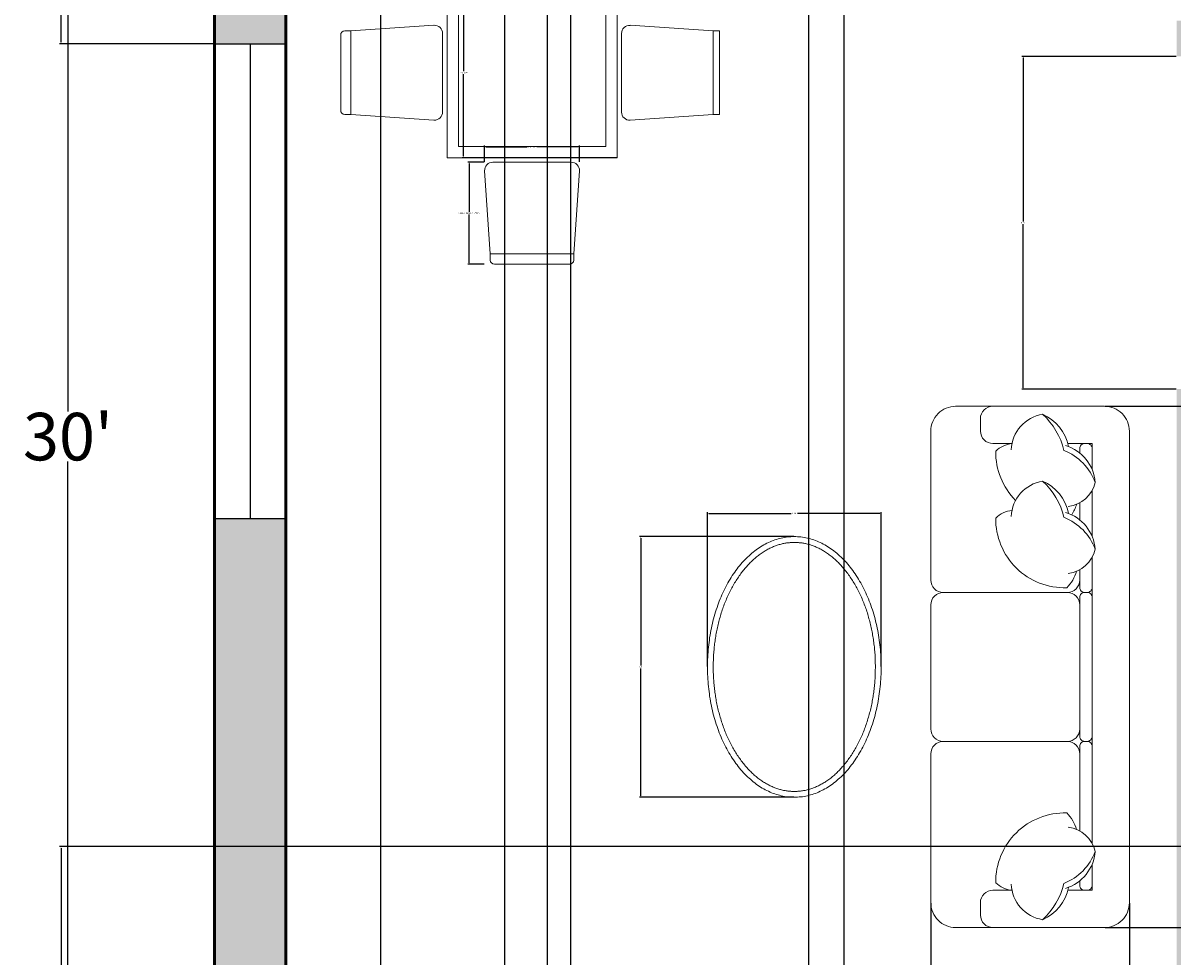
# Model space of a CAD drawing. Units: inches. Extents: x -2 to 282, y -370 to 35.
# Tile 2 of 5: x -2 to 143, y -237 to -119. Entities that reach past the tile are written whole.
import ezdxf

# ---------------------------------------------------------------- set-up
doc = ezdxf.new("R2010")
doc.units = ezdxf.units.IN
doc.header["$MEASUREMENT"] = 0
for name, color, linetype, lineweight in [('A-ANNO-DIMS', 2, 'Continuous', 18), ('A-FURN', 8, 'Continuous', 18), ('A-GLAZ', 4, 'Continuous', 25), ('A-WALL', 7, 'Continuous', 50), ('A-WALL-PATT', 252, 'Continuous', 13)]:
    doc.layers.add(name, color=color, linetype=linetype, lineweight=lineweight)
doc.styles.get("Standard").update_dxf_attribs({"font": 'arial.ttf'})
doc.dimstyles.get("Standard").update_dxf_attribs({"dimtxt": 0.18, "dimasz": 0.18, "dimexe": 0.18, "dimexo": 0.0625, "dimgap": 0.09, "dimtad": 0, "dimtih": 1, "dimtoh": 1, "dimdec": 0, "dimzin": 0, "dimdsep": 46, "dimlunit": 3, "dimtxsty": 'Standard', "dimcen": 0.09, "dimadec": 0, "dimazin": 0, "dimtfac": 1, "dimtdec": 0, "dimtofl": 0, "dimtmove": 0, "dimatfit": 3, "dimfxl": 1, "dimtolj": 1, "dimtzin": 0, "dimarcsym": 0})

# ---------------------------------------------------------------- blocks, each defined once
blk = doc.blocks.new('*D2')
at = {"layer": 'A-ANNO-DIMS', "color": 0, "lineweight": -2, "transparency": 16777216}
for p, q in [((22.35, 9.19), (3.74, 9.19)), ((3.92, 9.01), (3.92, -167.65)), ((3.92, -350.63), (3.92, -173.97)), ((22.35, -350.81), (3.74, -350.81))]:
    blk.add_line(p, q, dxfattribs=at)
at = {"layer": 'A-ANNO-DIMS', "color": 0, "transparency": 16777216}
for points in [[(3.89, 9.01), (3.95, 9.01), (3.92, 9.19)], [(3.89, -350.63), (3.95, -350.63), (3.92, -350.81)]]:
    blk.add_solid(points, dxfattribs=at)
at = {"layer": 'Defpoints', "color": 0, "transparency": 16777216}
for p in [(3.92, 9.19), (22.41, 9.19), (22.41, -350.81)]:
    blk.add_point(p, dxfattribs=at)
at = {"layer": 'A-ANNO-DIMS', "color": 0, "transparency": 16777216, "insert": (3.92, -170.81), "char_height": 6, "attachment_point": 5}
blk.add_mtext("\\A1;30'", dxfattribs=at)
blk = doc.blocks.new('WINDOW-60IN')
for p, q in [((0, 0), (0, 60)), ((0, 60), (9, 60)), ((4.5, 60), (4.5, 0)), ((9, 60), (9, 0)), ((9, 0), (0, 0))]:
    blk.add_line(p, q)
blk = doc.blocks.new('DINING-CHAIR')
for p, q in [((0.71, 12.36), (0.71, 11.58)), ((10.75, 12.87), (1.23, 12.87)), ((11.26, 11.58), (11.26, 12.36)), ((0, 1.09), (0.71, 11.58)), ((11.26, 11.58), (0.71, 11.58)), ((11.26, 11.58), (11.98, 1.09)), ((1.03, 0), (10.95, 0))]:
    blk.add_line(p, q)
for centre, radius, start, end in [((1.23, 12.36), 0.515, 90, 180), ((10.75, 12.36), 0.515, 0, 90), ((1.03, 1.03), 1.03, 176.8779, 270), ((10.95, 1.03), 1.03, 270, 3.1221)]:
    blk.add_arc(centre, radius, start, end)
blk = doc.blocks.new('*D15')
at = {"layer": 'A-ANNO-DIMS', "color": 0, "lineweight": -2, "transparency": 16777216}
for p, q in [((56.46, -136.16), (54.41, -136.16)), ((54.59, -136.34), (54.59, -142.42)), ((54.59, -148.86), (54.59, -142.78)), ((56.46, -149.04), (54.41, -149.04))]:
    blk.add_line(p, q, dxfattribs=at)
at = {"layer": 'A-ANNO-DIMS', "color": 0, "transparency": 16777216}
for points in [[(54.56, -136.34), (54.62, -136.34), (54.59, -136.16)], [(54.56, -148.86), (54.62, -148.86), (54.59, -149.04)]]:
    blk.add_solid(points, dxfattribs=at)
at = {"layer": 'Defpoints', "color": 0, "transparency": 16777216}
for p in [(56.52, -136.16), (54.59, -149.04), (56.52, -149.04)]:
    blk.add_point(p, dxfattribs=at)
at = {"layer": 'A-ANNO-DIMS', "color": 0, "transparency": 16777216, "insert": (54.59, -142.6), "char_height": 0.18, "attachment_point": 5}
blk.add_mtext('\\A1;DINING CHAIR 1\'-1" TYP.', dxfattribs=at)
blk = doc.blocks.new('*D16')
at = {"layer": 'A-ANNO-DIMS', "color": 0, "lineweight": -2, "transparency": 16777216}
for p, q in [((56.52, -136.1), (56.52, -134.05)), ((56.7, -134.23), (61.9, -134.23)), ((68.35, -134.23), (63.16, -134.23)), ((68.53, -136.1), (68.53, -134.05))]:
    blk.add_line(p, q, dxfattribs=at)
at = {"layer": 'A-ANNO-DIMS', "color": 0, "transparency": 16777216}
for points in [[(56.7, -134.2), (56.7, -134.26), (56.52, -134.23)], [(68.35, -134.2), (68.35, -134.26), (68.53, -134.23)]]:
    blk.add_solid(points, dxfattribs=at)
at = {"layer": 'Defpoints', "color": 0, "transparency": 16777216}
for p in [(56.52, -134.23), (56.52, -136.16), (68.53, -136.16)]:
    blk.add_point(p, dxfattribs=at)
at = {"layer": 'A-ANNO-DIMS', "color": 0, "transparency": 16777216, "insert": (62.53, -134.23), "char_height": 0.18, "attachment_point": 5}
blk.add_mtext('\\A1;1\'-0" TYP.', dxfattribs=at)
blk = doc.blocks.new('*D30')
at = {"layer": 'A-ANNO-DIMS', "color": 0, "lineweight": -2, "transparency": 16777216}
for p, q in [((22.35, -71.81), (2.86, -71.81)), ((3.04, -71.99), (3.04, -96.32)), ((3.04, -121.02), (3.04, -96.69)), ((22.35, -121.2), (2.86, -121.2))]:
    blk.add_line(p, q, dxfattribs=at)
at = {"layer": 'A-ANNO-DIMS', "color": 0, "transparency": 16777216}
for points in [[(3.01, -71.99), (3.07, -71.99), (3.04, -71.81)], [(3.01, -121.02), (3.07, -121.02), (3.04, -121.2)]]:
    blk.add_solid(points, dxfattribs=at)
at = {"layer": 'Defpoints', "color": 0, "transparency": 16777216}
for p in [(22.41, -71.81), (3.04, -121.2), (22.41, -121.2)]:
    blk.add_point(p, dxfattribs=at)
at = {"layer": 'A-ANNO-DIMS', "color": 0, "transparency": 16777216, "insert": (3.04, -96.51), "char_height": 0.18, "attachment_point": 5}
blk.add_mtext('\\A1;4\'-1 1/2"', dxfattribs=at)
blk = doc.blocks.new('*D37')
at = {"layer": 'A-ANNO-DIMS', "color": 0, "lineweight": -2, "transparency": 16777216}
for p, q in [((31.41, -277.25), (31.41, 28.74)), ((31.59, 28.56), (37.09, 28.56)), ((43.23, 28.56), (37.73, 28.56)), ((43.41, -277.25), (43.41, 28.74))]:
    blk.add_line(p, q, dxfattribs=at)
at = {"layer": 'A-ANNO-DIMS', "color": 0, "transparency": 16777216}
for points in [[(31.59, 28.59), (31.59, 28.53), (31.41, 28.56)], [(43.23, 28.59), (43.23, 28.53), (43.41, 28.56)]]:
    blk.add_solid(points, dxfattribs=at)
at = {"layer": 'Defpoints', "color": 0, "transparency": 16777216}
for p in [(43.41, 28.56), (31.41, -277.31), (43.41, -277.31)]:
    blk.add_point(p, dxfattribs=at)
at = {"layer": 'A-ANNO-DIMS', "color": 0, "transparency": 16777216, "insert": (37.41, 28.56), "char_height": 0.18, "attachment_point": 5}
blk.add_mtext('\\A1;1\'-0"', dxfattribs=at)
blk = doc.blocks.new('*D38')
at = {"layer": 'A-ANNO-DIMS', "color": 0, "lineweight": -2, "transparency": 16777216}
for p, q in [((43.41, -277.25), (43.41, 28.74)), ((43.59, 28.56), (55.08, 28.56)), ((67.23, 28.56), (55.74, 28.56)), ((67.41, -277.25), (67.41, 28.74))]:
    blk.add_line(p, q, dxfattribs=at)
at = {"layer": 'A-ANNO-DIMS', "color": 0, "transparency": 16777216}
for points in [[(43.59, 28.59), (43.59, 28.53), (43.41, 28.56)], [(67.23, 28.59), (67.23, 28.53), (67.41, 28.56)]]:
    blk.add_solid(points, dxfattribs=at)
at = {"layer": 'Defpoints', "color": 0, "transparency": 16777216}
for p in [(67.41, 28.56), (43.41, -277.31), (67.41, -277.31)]:
    blk.add_point(p, dxfattribs=at)
at = {"layer": 'A-ANNO-DIMS', "color": 0, "transparency": 16777216, "insert": (55.41, 28.56), "char_height": 0.18, "attachment_point": 5}
blk.add_mtext('\\A1;2\'-0"', dxfattribs=at)
blk = doc.blocks.new('*D39')
at = {"layer": 'A-ANNO-DIMS', "color": 0, "lineweight": -2, "transparency": 16777216}
for p, q in [((64.41, -88.37), (64.41, -370.37)), ((97.41, -88.37), (97.41, -370.37)), ((64.59, -370.19), (80.58, -370.19)), ((97.23, -370.19), (81.24, -370.19))]:
    blk.add_line(p, q, dxfattribs=at)
at = {"layer": 'A-ANNO-DIMS', "color": 0, "transparency": 16777216}
for points in [[(64.59, -370.16), (64.59, -370.22), (64.41, -370.19)], [(97.23, -370.16), (97.23, -370.22), (97.41, -370.19)]]:
    blk.add_solid(points, dxfattribs=at)
at = {"layer": 'Defpoints', "color": 0, "transparency": 16777216}
for p in [(64.41, -88.31), (97.41, -88.31), (97.41, -370.19)]:
    blk.add_point(p, dxfattribs=at)
at = {"layer": 'A-ANNO-DIMS', "color": 0, "transparency": 16777216, "insert": (80.91, -370.19), "char_height": 0.18, "attachment_point": 5}
blk.add_mtext('\\A1;2\'-9"', dxfattribs=at)
blk = doc.blocks.new('*D42')
at = {"layer": 'A-ANNO-DIMS', "color": 0, "lineweight": -2, "transparency": 16777216}
for p, q in [((31.41, -83.87), (31.41, -370.37)), ((59.05, -83.87), (59.05, -370.37)), ((31.59, -370.19), (44.69, -370.19)), ((58.87, -370.19), (45.77, -370.19))]:
    blk.add_line(p, q, dxfattribs=at)
at = {"layer": 'A-ANNO-DIMS', "color": 0, "transparency": 16777216}
for points in [[(31.59, -370.16), (31.59, -370.22), (31.41, -370.19)], [(58.87, -370.16), (58.87, -370.22), (59.05, -370.19)]]:
    blk.add_solid(points, dxfattribs=at)
at = {"layer": 'Defpoints', "color": 0, "transparency": 16777216}
for p in [(31.41, -83.81), (59.05, -83.81), (59.05, -370.19)]:
    blk.add_point(p, dxfattribs=at)
at = {"layer": 'A-ANNO-DIMS', "color": 0, "transparency": 16777216, "insert": (45.23, -370.19), "char_height": 0.18, "attachment_point": 5}
blk.add_mtext('\\A1;2\'-3 1/2"', dxfattribs=at)
blk = doc.blocks.new('*D46')
at = {"layer": 'A-ANNO-DIMS', "color": 0, "lineweight": -2, "transparency": 16777216}
for p, q in [((97.41, -88.37), (97.41, -370.37)), ((101.91, -88.37), (101.91, -370.37)), ((97.59, -370.19), (99.12, -370.19)), ((101.73, -370.19), (100.2, -370.19))]:
    blk.add_line(p, q, dxfattribs=at)
at = {"layer": 'A-ANNO-DIMS', "color": 0, "transparency": 16777216}
for points in [[(97.59, -370.16), (97.59, -370.22), (97.41, -370.19)], [(101.73, -370.16), (101.73, -370.22), (101.91, -370.19)]]:
    blk.add_solid(points, dxfattribs=at)
at = {"layer": 'Defpoints', "color": 0, "transparency": 16777216}
for p in [(97.41, -88.31), (101.91, -88.31), (101.91, -370.19)]:
    blk.add_point(p, dxfattribs=at)
at = {"layer": 'A-ANNO-DIMS', "color": 0, "transparency": 16777216, "insert": (99.66, -370.19), "char_height": 0.18, "attachment_point": 5}
blk.add_mtext('\\A1;0\'-4 1/2"', dxfattribs=at)
blk = doc.blocks.new('*D48')
at = {"layer": 'A-ANNO-DIMS', "color": 0, "lineweight": -2, "transparency": 16777216}
for p, q in [((112.88, -229.72), (112.88, -370.37)), ((137.95, -229.72), (137.95, -370.37)), ((113.06, -370.19), (125.08, -370.19)), ((137.77, -370.19), (125.74, -370.19))]:
    blk.add_line(p, q, dxfattribs=at)
at = {"layer": 'A-ANNO-DIMS', "color": 0, "transparency": 16777216}
for points in [[(113.06, -370.16), (113.06, -370.22), (112.88, -370.19)], [(137.77, -370.16), (137.77, -370.22), (137.95, -370.19)]]:
    blk.add_solid(points, dxfattribs=at)
at = {"layer": 'Defpoints', "color": 0, "transparency": 16777216}
for p in [(112.88, -229.66), (137.95, -229.66), (137.95, -370.19)]:
    blk.add_point(p, dxfattribs=at)
at = {"layer": 'A-ANNO-DIMS', "color": 0, "transparency": 16777216, "insert": (125.41, -370.19), "char_height": 0.18, "attachment_point": 5}
blk.add_mtext('\\A1;2\'-1"', dxfattribs=at)
blk = doc.blocks.new('*D49')
at = {"layer": 'A-ANNO-DIMS', "color": 0, "lineweight": -2, "transparency": 16777216}
for p, q in [((134.88, -166.98), (154.37, -166.98)), ((154.19, -167.16), (154.19, -199.71)), ((154.19, -232.61), (154.19, -200.07)), ((134.88, -232.79), (154.37, -232.79))]:
    blk.add_line(p, q, dxfattribs=at)
at = {"layer": 'A-ANNO-DIMS', "color": 0, "transparency": 16777216}
for points in [[(154.16, -167.16), (154.22, -167.16), (154.19, -166.98)], [(154.16, -232.61), (154.22, -232.61), (154.19, -232.79)]]:
    blk.add_solid(points, dxfattribs=at)
at = {"layer": 'Defpoints', "color": 0, "transparency": 16777216}
for p in [(134.81, -166.98), (134.81, -232.79), (154.19, -232.79)]:
    blk.add_point(p, dxfattribs=at)
at = {"layer": 'A-ANNO-DIMS', "color": 0, "transparency": 16777216, "insert": (154.19, -199.89), "char_height": 0.18, "attachment_point": 5}
blk.add_mtext('\\A1;5\'-6"', dxfattribs=at)
blk = doc.blocks.new('*D50')
at = {"layer": 'A-ANNO-DIMS', "color": 0, "lineweight": -2, "transparency": 16777216}
for p, q in [((73.19, -114.14), (53.7, -114.14)), ((53.88, -114.32), (53.88, -124.68)), ((53.88, -135.41), (53.88, -125.05)), ((73.19, -135.59), (53.7, -135.59))]:
    blk.add_line(p, q, dxfattribs=at)
at = {"layer": 'A-ANNO-DIMS', "color": 0, "transparency": 16777216}
for points in [[(53.85, -114.32), (53.91, -114.32), (53.88, -114.14)], [(53.85, -135.41), (53.91, -135.41), (53.88, -135.59)]]:
    blk.add_solid(points, dxfattribs=at)
at = {"layer": 'Defpoints', "color": 0, "transparency": 16777216}
for p in [(53.88, -114.14), (73.25, -114.14), (73.25, -135.59)]:
    blk.add_point(p, dxfattribs=at)
at = {"layer": 'A-ANNO-DIMS', "color": 0, "transparency": 16777216, "insert": (53.88, -124.87), "char_height": 0.18, "attachment_point": 5}
blk.add_mtext('\\A1;1\'-9 1/2"', dxfattribs=at)
blk = doc.blocks.new('*D53')
at = {"layer": 'A-ANNO-DIMS', "color": 0, "lineweight": -2, "transparency": 16777216}
for p, q in [((185.51, -222.58), (2.86, -222.58)), ((3.04, -222.76), (3.04, -242.71)), ((3.04, -263.02), (3.04, -243.07)), ((185.51, -263.2), (2.86, -263.2))]:
    blk.add_line(p, q, dxfattribs=at)
at = {"layer": 'A-ANNO-DIMS', "color": 0, "transparency": 16777216}
for points in [[(3.01, -222.76), (3.07, -222.76), (3.04, -222.58)], [(3.01, -263.02), (3.07, -263.02), (3.04, -263.2)]]:
    blk.add_solid(points, dxfattribs=at)
at = {"layer": 'Defpoints', "color": 0, "transparency": 16777216}
for p in [(3.04, -222.58), (185.58, -222.58), (185.58, -263.2)]:
    blk.add_point(p, dxfattribs=at)
at = {"layer": 'A-ANNO-DIMS', "color": 0, "transparency": 16777216, "insert": (3.04, -242.89), "char_height": 0.18, "attachment_point": 5}
blk.add_mtext('\\A1;3\'-4 1/2"', dxfattribs=at)
blk = doc.blocks.new('*D56')
at = {"layer": 'A-ANNO-DIMS', "color": 0, "lineweight": -2, "transparency": 16777216}
for p, q in [((84.67, -199.83), (84.67, -180.33)), ((84.85, -180.51), (95.25, -180.51)), ((106.43, -180.51), (96.03, -180.51)), ((106.61, -199.83), (106.61, -180.33))]:
    blk.add_line(p, q, dxfattribs=at)
at = {"layer": 'A-ANNO-DIMS', "color": 0, "transparency": 16777216}
for points in [[(84.85, -180.48), (84.85, -180.54), (84.67, -180.51)], [(106.43, -180.48), (106.43, -180.54), (106.61, -180.51)]]:
    blk.add_solid(points, dxfattribs=at)
at = {"layer": 'Defpoints', "color": 0, "transparency": 16777216}
for p in [(106.61, -180.51), (84.67, -199.89), (106.61, -199.89)]:
    blk.add_point(p, dxfattribs=at)
at = {"layer": 'A-ANNO-DIMS', "color": 0, "transparency": 16777216, "insert": (95.64, -180.51), "char_height": 0.18, "attachment_point": 5}
blk.add_mtext('\\A1;1\'-10"', dxfattribs=at)
blk = doc.blocks.new('*D57')
at = {"layer": 'A-ANNO-DIMS', "color": 0, "lineweight": -2, "transparency": 16777216}
for p, q in [((95.58, -183.43), (76.08, -183.43)), ((76.26, -183.61), (76.26, -199.71)), ((76.26, -216.16), (76.26, -200.07)), ((95.58, -216.34), (76.08, -216.34))]:
    blk.add_line(p, q, dxfattribs=at)
at = {"layer": 'A-ANNO-DIMS', "color": 0, "transparency": 16777216}
for points in [[(76.23, -183.61), (76.29, -183.61), (76.26, -183.43)], [(76.23, -216.16), (76.29, -216.16), (76.26, -216.34)]]:
    blk.add_solid(points, dxfattribs=at)
at = {"layer": 'Defpoints', "color": 0, "transparency": 16777216}
for p in [(76.26, -183.43), (95.64, -183.43), (95.64, -216.34)]:
    blk.add_point(p, dxfattribs=at)
at = {"layer": 'A-ANNO-DIMS', "color": 0, "transparency": 16777216, "insert": (76.26, -199.89), "char_height": 0.18, "attachment_point": 5}
blk.add_mtext('\\A1;2\'-9"', dxfattribs=at)
blk = doc.blocks.new('*D59')
at = {"layer": 'A-ANNO-DIMS', "color": 0, "lineweight": -2, "transparency": 16777216}
for p, q in [((143.85, -122.81), (124.36, -122.81)), ((124.54, -122.99), (124.54, -143.63)), ((124.54, -164.63), (124.54, -143.99)), ((143.85, -164.81), (124.36, -164.81))]:
    blk.add_line(p, q, dxfattribs=at)
at = {"layer": 'A-ANNO-DIMS', "color": 0, "transparency": 16777216}
for points in [[(124.51, -122.99), (124.57, -122.99), (124.54, -122.81)], [(124.51, -164.63), (124.57, -164.63), (124.54, -164.81)]]:
    blk.add_solid(points, dxfattribs=at)
at = {"layer": 'Defpoints', "color": 0, "transparency": 16777216}
for p in [(124.54, -122.81), (143.91, -122.81), (143.91, -164.81)]:
    blk.add_point(p, dxfattribs=at)
at = {"layer": 'A-ANNO-DIMS', "color": 0, "transparency": 16777216, "insert": (124.54, -143.81), "char_height": 0.18, "attachment_point": 5}
blk.add_mtext('\\A1;3\'-6"', dxfattribs=at)

msp = doc.modelspace()

# ---------------------------------------------------------------- hatches: boundary and pattern name
at = {"layer": 'A-WALL-PATT'}
h = msp.add_hatch(color=256, dxfattribs=at)
h.dxf.hatch_style = 1
h.paths.add_polyline_path([(262.41, 9.19), (134.91, 9.19), (134.91, 0.19), (143.91, 0.19), (143.91, -35.81), (148.41, -35.81), (148.41, 0.19), (253.41, 0.19), (253.41, -29.06), (262.41, -29.06)])
h.paths.add_polyline_path([(110.91, 9.19), (22.41, 9.19), (22.41, -11.81), (31.41, -11.81), (31.41, 0.19), (97.41, 0.19), (97.41, -88.31), (101.91, -88.31), (101.91, -64.31), (143.91, -64.31), (143.91, -88.31), (148.41, -88.31), (148.41, -59.81), (101.91, -59.81), (101.91, 0.19), (110.91, 0.19)])
h.paths.add_polyline_path([(31.41, -88.31), (64.41, -88.31), (64.41, -83.81), (31.41, -83.81), (31.41, -71.81), (22.41, -71.81), (22.41, -121.2), (31.41, -121.2)])
h.paths.add_polyline_path([(262.41, -89.06), (253.41, -89.06), (253.41, -118.31), (143.91, -118.31), (143.91, -122.81), (184.41, -122.81), (184.41, -164.81), (184.41, -169.31), (188.91, -169.31), (188.91, -164.81), (188.91, -122.81), (253.41, -122.81), (253.41, -131.81), (262.41, -131.81)])
h.paths.add_polyline_path([(262.41, -155.81), (253.41, -155.81), (253.41, -164.81), (212.91, -164.81), (212.91, -169.31), (253.41, -169.31), (253.41, -193.31), (262.41, -193.31)])
h.paths.add_polyline_path([(262.41, -253.31), (253.41, -253.31), (253.41, -277.31), (148.41, -277.31), (148.41, -164.81), (143.91, -164.81), (143.91, -169.31), (143.91, -281.81), (253.41, -281.81), (253.41, -341.81), (143.91, -341.81), (143.91, -350.81), (262.41, -350.81)])
h.paths.add_polyline_path([(31.41, -323.81), (22.41, -323.81), (22.41, -350.81), (95.91, -350.81), (95.91, -281.81), (107.91, -281.81), (107.91, -277.31), (67.41, -277.31), (67.41, -281.81), (91.41, -281.81), (91.41, -341.81), (31.41, -341.81)])
h.paths.add_polyline_path([(43.41, -277.31), (31.41, -277.31), (31.41, -181.2), (22.41, -181.2), (22.41, -299.81), (31.41, -299.81), (31.41, -281.81), (43.41, -281.81)])

# ---------------------------------------------------------------- linework, layer by layer
at = {"layer": 'A-FURN'}
for p, q in [((74.91, -118.88), (85.41, -119.59)), ((73.82, -119.91), (73.82, -129.83)), ((86.18, -119.59), (85.41, -119.59)), ((85.41, -130.14), (85.41, -119.59)), ((86.18, -119.59), (86.18, -130.14)), ((85.41, -130.14), (74.91, -130.86)), ((85.41, -130.14), (86.18, -130.14))]:
    msp.add_line(p, q, dxfattribs=at)
for points in [[(51.8, -135.59), (51.8, -114.14), (73.25, -114.14), (73.25, -135.59)], [(53.23, -134.16), (53.23, -115.57), (71.82, -115.57), (71.82, -134.16)]]:
    msp.add_lwpolyline(points, close=True, dxfattribs=at)
at = {"layer": 'A-FURN', "ltscale": 0.03}
msp.add_lwpolyline([(116.01, -232.79, -0.414214), (112.88, -229.66), (112.88, -210.86, -0.414214), (114.44, -209.29, -0.414214), (112.88, -207.72), (112.88, -192.05, -0.414214), (114.44, -190.49, -0.414214), (112.88, -188.92), (112.88, -170.12, -0.414214), (116.01, -166.98), (134.81, -166.98, -0.414214), (137.95, -170.12), (137.95, -229.66, -0.414214), (134.81, -232.79)], format="xyb", close=True, dxfattribs=at)
at = {"layer": 'A-FURN'}
for points in [[(123.14, -171.68), (120.71, -171.68, -0.414214), (119.14, -170.12), (119.14, -168.55, -0.414214), (120.71, -166.98)], [(123.04, -172.47, -0.356772), (126.99, -167.98, -0.249542), (130.25, -172.05, 9.61688)], [(126.99, -167.98, -0.14773), (129.69, -172.56, -0.213343), (133.64, -176.6, -0.178662)], [(123.14, -171.68, 0.165541), (121.07, -172.65, 0.200231), (123.59, -178.87, 0.121523)], [(129.9, -171.93, -0.306663), (133.64, -176.6, -0.30633), (130.23, -179.65, 0.872847)], [(133.25, -174.98), (133.25, -171.68), (130.17, -171.68, -0.414214)], [(131.68, -172.88), (131.68, -172.31, -0.414214), (132.31, -171.68), (132.62, -171.68, -0.414214), (133.25, -172.31)], [(133.25, -172.31), (133.25, -174.98, -0.414214)], [(123.04, -180.91, -0.356772), (126.99, -176.42, -0.249542), (130.25, -180.49, 9.61688)], [(126.99, -176.42, -0.14773), (129.69, -181, -0.213343), (133.64, -185.04, -0.178662)], [(133.25, -177.59), (133.25, -183.42, -0.414214)], [(130.67, -180.67, 0.071865), (131.28, -179.36, -7.115464)], [(131.68, -181.32), (131.68, -179.16, -0.414214)], [(123.14, -180.12, 0.165541), (121.07, -181.09, 0.425989), (130.05, -189.89, 0.121523), (131.28, -187.8, -7.115464)], [(129.9, -180.37, -0.306663), (133.64, -185.04, -0.30633), (130.23, -188.09, 0.872847)], [(133.25, -186.03), (133.25, -189.86, -0.414214), (132.62, -190.49), (132.31, -190.49, -0.414214), (131.68, -189.86), (131.68, -187.6, -0.414214)], [(131.68, -188.92, -0.414214), (130.11, -190.49), (114.44, -190.49, -0.414214)], [(131.68, -192.05, 0.414214), (130.11, -190.49)], [(131.68, -207.72, -0.414214), (130.11, -209.29)], [(131.68, -210.86, 0.414214), (130.11, -209.29), (114.44, -209.29, 0.414214)], [(133.25, -222.19), (133.25, -209.92, 0.414214), (132.62, -209.29), (132.31, -209.29, 0.414214), (131.68, -209.92), (131.68, -220.61, 0.414214)], [(123.14, -228.1, -0.165541), (121.07, -227.13, -0.425989), (130.05, -218.33, -0.121523), (131.28, -220.42, 7.115464)], [(129.9, -227.85, 0.306663), (133.64, -223.18, 0.30633), (130.23, -220.12, -0.872847)], [(126.99, -231.8, 0.14773), (129.69, -227.22, 0.213343), (133.64, -223.18, 0.178662)], [(133.25, -227.47), (133.25, -224.8, 0.414214)], [(123.04, -227.31, 0.356772), (126.99, -231.8, 0.249542), (130.25, -227.73, -9.61688)], [(131.68, -226.9), (131.68, -227.47, 0.414214), (132.31, -228.09), (132.62, -228.09, 0.414214), (133.25, -227.47)], [(120.71, -232.79, -0.414214), (119.14, -231.23), (119.14, -229.66, -0.414214), (120.71, -228.09), (123.14, -228.09)]]:
    msp.add_lwpolyline(points, format="xyb", dxfattribs=at)
for points in [[(133.25, -183.42), (133.25, -177.59)], [(133.25, -222.19), (133.25, -186.03)], [(130.17, -228.09), (133.25, -228.09), (133.25, -224.8)]]:
    msp.add_lwpolyline(points, dxfattribs=at)
msp.add_lwpolyline([(133.25, -191.11), (133.25, -208.66, -0.414214), (132.62, -209.29), (132.31, -209.29, -0.414214), (131.68, -208.66), (131.68, -191.11, -0.414214), (132.31, -190.49), (132.62, -190.49, -0.414214)], format="xyb", close=True, dxfattribs=at)
at = {"layer": 'A-FURN', "ltscale": 0.03}
msp.add_polyline3d([(95.64, -216.34, 0), (95.85, -216.34, 0), (96.05, -216.33, 0), (96.26, -216.31, 0), (96.47, -216.29, 0), (96.68, -216.27, 0), (96.88, -216.24, 0), (97.09, -216.2, 0), (97.29, -216.15, 0), (97.5, -216.1, 0), (97.7, -216.05, 0), (97.91, -215.99, 0), (98.11, -215.92, 0), (98.31, -215.85, 0), (98.51, -215.77, 0), (98.71, -215.68, 0), (98.91, -215.59, 0), (99.11, -215.5, 0), (99.3, -215.4, 0), (99.5, -215.29, 0), (99.69, -215.18, 0), (99.88, -215.06, 0), (100.08, -214.94, 0), (100.26, -214.81, 0), (100.45, -214.67, 0), (100.64, -214.53, 0), (100.82, -214.39, 0), (101, -214.24, 0), (101.18, -214.08, 0), (101.36, -213.92, 0), (101.54, -213.76, 0), (101.71, -213.59, 0), (101.88, -213.42, 0), (102.05, -213.24, 0), (102.22, -213.05, 0), (102.39, -212.86, 0), (102.55, -212.67, 0), (102.71, -212.47, 0), (102.87, -212.27, 0), (103.02, -212.06, 0), (103.17, -211.85, 0), (103.32, -211.63, 0), (103.47, -211.41, 0), (103.61, -211.19, 0), (103.75, -210.96, 0), (103.89, -210.73, 0), (104.03, -210.49, 0), (104.16, -210.25, 0), (104.29, -210.01, 0), (104.41, -209.76, 0), (104.54, -209.51, 0), (104.66, -209.25, 0), (104.77, -209, 0), (104.89, -208.74, 0), (105, -208.47, 0), (105.1, -208.2, 0), (105.21, -207.93, 0), (105.31, -207.66, 0), (105.4, -207.39, 0), (105.5, -207.11, 0), (105.59, -206.83, 0), (105.67, -206.54, 0), (105.75, -206.26, 0), (105.83, -205.97, 0), (105.91, -205.68, 0), (105.98, -205.38, 0), (106.05, -205.09, 0), (106.11, -204.79, 0), (106.17, -204.5, 0), (106.23, -204.2, 0), (106.28, -203.9, 0), (106.33, -203.59, 0), (106.37, -203.29, 0), (106.41, -202.98, 0), (106.45, -202.68, 0), (106.48, -202.37, 0), (106.51, -202.06, 0), (106.54, -201.75, 0), (106.56, -201.44, 0), (106.58, -201.13, 0), (106.59, -200.82, 0), (106.6, -200.51, 0), (106.61, -200.2, 0), (106.61, -199.89, 0), (106.61, -199.58, 0), (106.6, -199.27, 0), (106.59, -198.95, 0), (106.58, -198.64, 0), (106.56, -198.33, 0), (106.54, -198.02, 0), (106.51, -197.71, 0), (106.48, -197.41, 0), (106.45, -197.1, 0), (106.41, -196.79, 0), (106.37, -196.49, 0), (106.33, -196.18, 0), (106.28, -195.88, 0), (106.23, -195.58, 0), (106.17, -195.28, 0), (106.11, -194.98, 0), (106.05, -194.69, 0), (105.98, -194.39, 0), (105.91, -194.1, 0), (105.83, -193.81, 0), (105.75, -193.52, 0), (105.67, -193.23, 0), (105.59, -192.95, 0), (105.5, -192.67, 0), (105.4, -192.39, 0), (105.31, -192.11, 0), (105.21, -191.84, 0), (105.1, -191.57, 0), (105, -191.3, 0), (104.89, -191.04, 0), (104.77, -190.78, 0), (104.66, -190.52, 0), (104.54, -190.27, 0), (104.41, -190.02, 0), (104.29, -189.77, 0), (104.16, -189.53, 0), (104.03, -189.29, 0), (103.89, -189.05, 0), (103.75, -188.82, 0), (103.61, -188.59, 0), (103.47, -188.36, 0), (103.32, -188.14, 0), (103.17, -187.93, 0), (103.02, -187.72, 0), (102.87, -187.51, 0), (102.71, -187.31, 0), (102.55, -187.11, 0), (102.39, -186.91, 0), (102.22, -186.72, 0), (102.05, -186.54, 0), (101.88, -186.36, 0), (101.71, -186.19, 0), (101.54, -186.02, 0), (101.36, -185.85, 0), (101.18, -185.69, 0), (101, -185.54, 0), (100.82, -185.39, 0), (100.64, -185.24, 0), (100.45, -185.1, 0), (100.26, -184.97, 0), (100.08, -184.84, 0), (99.88, -184.72, 0), (99.69, -184.6, 0), (99.5, -184.49, 0), (99.3, -184.38, 0), (99.11, -184.28, 0), (98.91, -184.18, 0), (98.71, -184.09, 0), (98.51, -184.01, 0), (98.31, -183.93, 0), (98.11, -183.86, 0), (97.91, -183.79, 0), (97.7, -183.73, 0), (97.5, -183.67, 0), (97.29, -183.62, 0), (97.09, -183.58, 0), (96.88, -183.54, 0), (96.68, -183.51, 0), (96.47, -183.48, 0), (96.26, -183.46, 0), (96.05, -183.45, 0), (95.85, -183.44, 0), (95.64, -183.43, 0), (95.43, -183.44, 0), (95.22, -183.45, 0), (95.02, -183.46, 0), (94.81, -183.48, 0), (94.6, -183.51, 0), (94.4, -183.54, 0), (94.19, -183.58, 0), (93.98, -183.62, 0), (93.78, -183.67, 0), (93.58, -183.73, 0), (93.37, -183.79, 0), (93.17, -183.86, 0), (92.97, -183.93, 0), (92.77, -184.01, 0), (92.57, -184.09, 0), (92.37, -184.18, 0), (92.17, -184.28, 0), (91.97, -184.38, 0), (91.78, -184.49, 0), (91.59, -184.6, 0), (91.39, -184.72, 0), (91.2, -184.84, 0), (91.01, -184.97, 0), (90.83, -185.1, 0), (90.64, -185.24, 0), (90.46, -185.39, 0), (90.28, -185.54, 0), (90.1, -185.69, 0), (89.92, -185.85, 0), (89.74, -186.02, 0), (89.57, -186.19, 0), (89.4, -186.36, 0), (89.23, -186.54, 0), (89.06, -186.72, 0), (88.89, -186.91, 0), (88.73, -187.11, 0), (88.57, -187.31, 0), (88.41, -187.51, 0), (88.26, -187.72, 0), (88.11, -187.93, 0), (87.96, -188.14, 0), (87.81, -188.36, 0), (87.67, -188.59, 0), (87.52, -188.82, 0), (87.39, -189.05, 0), (87.25, -189.29, 0), (87.12, -189.53, 0), (86.99, -189.77, 0), (86.86, -190.02, 0), (86.74, -190.27, 0), (86.62, -190.52, 0), (86.5, -190.78, 0), (86.39, -191.04, 0), (86.28, -191.3, 0), (86.17, -191.57, 0), (86.07, -191.84, 0), (85.97, -192.11, 0), (85.88, -192.39, 0), (85.78, -192.67, 0), (85.69, -192.95, 0), (85.61, -193.23, 0), (85.53, -193.52, 0), (85.45, -193.81, 0), (85.37, -194.1, 0), (85.3, -194.39, 0), (85.23, -194.69, 0), (85.17, -194.98, 0), (85.11, -195.28, 0), (85.05, -195.58, 0), (85, -195.88, 0), (84.95, -196.18, 0), (84.91, -196.49, 0), (84.87, -196.79, 0), (84.83, -197.1, 0), (84.8, -197.41, 0), (84.77, -197.71, 0), (84.74, -198.02, 0), (84.72, -198.33, 0), (84.7, -198.64, 0), (84.69, -198.95, 0), (84.68, -199.27, 0), (84.67, -199.58, 0), (84.67, -199.89, 0), (84.67, -200.2, 0), (84.68, -200.51, 0), (84.69, -200.82, 0), (84.7, -201.13, 0), (84.72, -201.44, 0), (84.74, -201.75, 0), (84.77, -202.06, 0), (84.8, -202.37, 0), (84.83, -202.68, 0), (84.87, -202.98, 0), (84.91, -203.29, 0), (84.95, -203.59, 0), (85, -203.9, 0), (85.05, -204.2, 0), (85.11, -204.5, 0), (85.17, -204.79, 0), (85.23, -205.09, 0), (85.3, -205.38, 0), (85.37, -205.68, 0), (85.45, -205.97, 0), (85.53, -206.26, 0), (85.61, -206.54, 0), (85.69, -206.83, 0), (85.78, -207.11, 0), (85.88, -207.39, 0), (85.97, -207.66, 0), (86.07, -207.93, 0), (86.17, -208.2, 0), (86.28, -208.47, 0), (86.39, -208.74, 0), (86.5, -209, 0), (86.62, -209.25, 0), (86.74, -209.51, 0), (86.86, -209.76, 0), (86.99, -210.01, 0), (87.12, -210.25, 0), (87.25, -210.49, 0), (87.39, -210.73, 0), (87.52, -210.96, 0), (87.67, -211.19, 0), (87.81, -211.41, 0), (87.96, -211.63, 0), (88.11, -211.85, 0), (88.26, -212.06, 0), (88.41, -212.27, 0), (88.57, -212.47, 0), (88.73, -212.67, 0), (88.89, -212.86, 0), (89.06, -213.05, 0), (89.23, -213.24, 0), (89.4, -213.42, 0), (89.57, -213.59, 0), (89.74, -213.76, 0), (89.92, -213.92, 0), (90.1, -214.08, 0), (90.28, -214.24, 0), (90.46, -214.39, 0), (90.64, -214.53, 0), (90.83, -214.67, 0), (91.01, -214.81, 0), (91.2, -214.94, 0), (91.39, -215.06, 0), (91.59, -215.18, 0), (91.78, -215.29, 0), (91.97, -215.4, 0), (92.17, -215.5, 0), (92.37, -215.59, 0), (92.57, -215.68, 0), (92.77, -215.77, 0), (92.97, -215.85, 0), (93.17, -215.92, 0), (93.37, -215.99, 0), (93.58, -216.05, 0), (93.78, -216.1, 0), (93.98, -216.15, 0), (94.19, -216.2, 0), (94.4, -216.24, 0), (94.6, -216.27, 0), (94.81, -216.29, 0), (95.02, -216.31, 0), (95.22, -216.33, 0), (95.43, -216.34, 0), (95.64, -216.34, 0)], dxfattribs=at)
at = {"layer": 'A-FURN'}
msp.add_polyline3d([(95.64, -215.61, 0), (95.75, -215.61, 0), (95.86, -215.61, 0), (95.98, -215.6, 0), (96.09, -215.59, 0), (96.21, -215.59, 0), (96.32, -215.57, 0), (96.43, -215.56, 0), (96.55, -215.55, 0), (96.67, -215.53, 0), (96.78, -215.51, 0), (96.9, -215.49, 0), (97.02, -215.47, 0), (97.13, -215.44, 0), (97.25, -215.41, 0), (97.37, -215.38, 0), (97.49, -215.35, 0), (97.61, -215.31, 0), (97.72, -215.28, 0), (97.84, -215.24, 0), (97.96, -215.19, 0), (98.08, -215.15, 0), (98.2, -215.1, 0), (98.32, -215.05, 0), (98.44, -215, 0), (98.56, -214.95, 0), (98.68, -214.89, 0), (98.8, -214.83, 0), (98.92, -214.77, 0), (99.04, -214.71, 0), (99.16, -214.64, 0), (99.28, -214.57, 0), (99.4, -214.5, 0), (99.52, -214.42, 0), (99.64, -214.35, 0), (99.76, -214.27, 0), (99.88, -214.18, 0), (100, -214.1, 0), (100.11, -214.01, 0), (100.23, -213.92, 0), (100.35, -213.83, 0), (100.47, -213.74, 0), (100.58, -213.64, 0), (100.7, -213.54, 0), (100.81, -213.44, 0), (100.93, -213.33, 0), (101.04, -213.22, 0), (101.15, -213.11, 0), (101.26, -213, 0), (101.38, -212.88, 0), (101.49, -212.76, 0), (101.6, -212.64, 0), (101.7, -212.52, 0), (101.81, -212.4, 0), (101.92, -212.27, 0), (102.03, -212.14, 0), (102.13, -212, 0), (102.24, -211.87, 0), (102.34, -211.73, 0), (102.44, -211.59, 0), (102.54, -211.45, 0), (102.64, -211.31, 0), (102.74, -211.16, 0), (102.84, -211.02, 0), (102.94, -210.87, 0), (103.03, -210.72, 0), (103.13, -210.56, 0), (103.22, -210.41, 0), (103.31, -210.25, 0), (103.4, -210.09, 0), (103.49, -209.93, 0), (103.58, -209.77, 0), (103.67, -209.61, 0), (103.75, -209.44, 0), (103.83, -209.27, 0), (103.92, -209.11, 0), (104, -208.94, 0), (104.07, -208.77, 0), (104.15, -208.59, 0), (104.23, -208.42, 0), (104.3, -208.24, 0), (104.37, -208.07, 0), (104.44, -207.89, 0), (104.51, -207.71, 0), (104.58, -207.53, 0), (104.64, -207.35, 0), (104.71, -207.17, 0), (104.77, -206.98, 0), (104.83, -206.8, 0), (104.88, -206.62, 0), (104.94, -206.44, 0), (105, -206.25, 0), (105.05, -206.07, 0), (105.1, -205.88, 0), (105.15, -205.7, 0), (105.2, -205.51, 0), (105.24, -205.33, 0), (105.29, -205.14, 0), (105.33, -204.96, 0), (105.37, -204.77, 0), (105.41, -204.58, 0), (105.45, -204.39, 0), (105.48, -204.21, 0), (105.52, -204.02, 0), (105.55, -203.83, 0), (105.58, -203.64, 0), (105.61, -203.45, 0), (105.64, -203.27, 0), (105.67, -203.08, 0), (105.69, -202.89, 0), (105.71, -202.7, 0), (105.74, -202.51, 0), (105.76, -202.32, 0), (105.77, -202.13, 0), (105.79, -201.94, 0), (105.81, -201.75, 0), (105.82, -201.56, 0), (105.83, -201.37, 0), (105.84, -201.18, 0), (105.85, -200.99, 0), (105.86, -200.79, 0), (105.87, -200.6, 0), (105.87, -200.41, 0), (105.87, -200.22, 0), (105.88, -200.03, 0), (105.88, -199.84, 0), (105.88, -199.65, 0), (105.87, -199.46, 0), (105.87, -199.27, 0), (105.86, -199.08, 0), (105.86, -198.89, 0), (105.85, -198.7, 0), (105.84, -198.5, 0), (105.83, -198.31, 0), (105.81, -198.12, 0), (105.8, -197.93, 0), (105.78, -197.74, 0), (105.76, -197.55, 0), (105.75, -197.36, 0), (105.72, -197.17, 0), (105.7, -196.98, 0), (105.68, -196.79, 0), (105.65, -196.61, 0), (105.63, -196.42, 0), (105.6, -196.23, 0), (105.57, -196.04, 0), (105.53, -195.85, 0), (105.5, -195.66, 0), (105.47, -195.47, 0), (105.43, -195.29, 0), (105.39, -195.1, 0), (105.35, -194.91, 0), (105.31, -194.73, 0), (105.26, -194.54, 0), (105.22, -194.36, 0), (105.17, -194.17, 0), (105.12, -193.98, 0), (105.07, -193.8, 0), (105.02, -193.62, 0), (104.97, -193.43, 0), (104.91, -193.25, 0), (104.86, -193.07, 0), (104.8, -192.88, 0), (104.74, -192.7, 0), (104.67, -192.52, 0), (104.61, -192.34, 0), (104.54, -192.16, 0), (104.48, -191.98, 0), (104.41, -191.8, 0), (104.34, -191.62, 0), (104.26, -191.45, 0), (104.19, -191.27, 0), (104.11, -191.1, 0), (104.03, -190.92, 0), (103.96, -190.75, 0), (103.87, -190.59, 0), (103.79, -190.42, 0), (103.71, -190.25, 0), (103.62, -190.09, 0), (103.54, -189.92, 0), (103.45, -189.76, 0), (103.36, -189.6, 0), (103.27, -189.45, 0), (103.17, -189.29, 0), (103.08, -189.14, 0), (102.99, -188.98, 0), (102.89, -188.83, 0), (102.79, -188.69, 0), (102.69, -188.54, 0), (102.59, -188.39, 0), (102.49, -188.25, 0), (102.39, -188.11, 0), (102.29, -187.97, 0), (102.18, -187.84, 0), (102.08, -187.7, 0), (101.97, -187.57, 0), (101.87, -187.44, 0), (101.76, -187.32, 0), (101.65, -187.19, 0), (101.54, -187.07, 0), (101.43, -186.95, 0), (101.32, -186.83, 0), (101.21, -186.72, 0), (101.1, -186.61, 0), (100.98, -186.5, 0), (100.87, -186.39, 0), (100.75, -186.29, 0), (100.64, -186.19, 0), (100.52, -186.09, 0), (100.41, -185.99, 0), (100.29, -185.9, 0), (100.17, -185.81, 0), (100.06, -185.72, 0), (99.94, -185.63, 0), (99.82, -185.55, 0), (99.7, -185.47, 0), (99.58, -185.39, 0), (99.46, -185.32, 0), (99.34, -185.24, 0), (99.22, -185.17, 0), (99.1, -185.1, 0), (98.98, -185.04, 0), (98.86, -184.98, 0), (98.74, -184.91, 0), (98.62, -184.86, 0), (98.5, -184.8, 0), (98.38, -184.75, 0), (98.26, -184.7, 0), (98.14, -184.65, 0), (98.02, -184.6, 0), (97.9, -184.56, 0), (97.78, -184.52, 0), (97.67, -184.48, 0), (97.55, -184.44, 0), (97.43, -184.41, 0), (97.31, -184.38, 0), (97.19, -184.35, 0), (97.07, -184.32, 0), (96.96, -184.3, 0), (96.84, -184.28, 0), (96.72, -184.26, 0), (96.61, -184.24, 0), (96.49, -184.22, 0), (96.38, -184.21, 0), (96.26, -184.2, 0), (96.15, -184.19, 0), (96.03, -184.18, 0), (95.92, -184.17, 0), (95.81, -184.17, 0), (95.7, -184.17, 0), (95.58, -184.17, 0), (95.47, -184.17, 0), (95.36, -184.17, 0), (95.24, -184.18, 0), (95.13, -184.19, 0), (95.02, -184.2, 0), (94.9, -184.21, 0), (94.79, -184.22, 0), (94.67, -184.24, 0), (94.55, -184.26, 0), (94.44, -184.28, 0), (94.32, -184.3, 0), (94.2, -184.32, 0), (94.09, -184.35, 0), (93.97, -184.38, 0), (93.85, -184.41, 0), (93.73, -184.44, 0), (93.61, -184.48, 0), (93.49, -184.52, 0), (93.37, -184.56, 0), (93.26, -184.6, 0), (93.14, -184.65, 0), (93.02, -184.7, 0), (92.9, -184.75, 0), (92.78, -184.8, 0), (92.66, -184.86, 0), (92.54, -184.91, 0), (92.42, -184.98, 0), (92.3, -185.04, 0), (92.18, -185.1, 0), (92.06, -185.17, 0), (91.94, -185.24, 0), (91.82, -185.32, 0), (91.7, -185.39, 0), (91.58, -185.47, 0), (91.46, -185.55, 0), (91.34, -185.63, 0), (91.22, -185.72, 0), (91.11, -185.81, 0), (90.99, -185.9, 0), (90.87, -185.99, 0), (90.76, -186.09, 0), (90.64, -186.19, 0), (90.52, -186.29, 0), (90.41, -186.39, 0), (90.3, -186.5, 0), (90.18, -186.61, 0), (90.07, -186.72, 0), (89.96, -186.83, 0), (89.85, -186.95, 0), (89.74, -187.07, 0), (89.63, -187.19, 0), (89.52, -187.32, 0), (89.41, -187.44, 0), (89.31, -187.57, 0), (89.2, -187.7, 0), (89.09, -187.84, 0), (88.99, -187.97, 0), (88.89, -188.11, 0), (88.79, -188.25, 0), (88.68, -188.39, 0), (88.59, -188.54, 0), (88.49, -188.69, 0), (88.39, -188.83, 0), (88.29, -188.98, 0), (88.2, -189.14, 0), (88.1, -189.29, 0), (88.01, -189.45, 0), (87.92, -189.6, 0), (87.83, -189.76, 0), (87.74, -189.92, 0), (87.66, -190.09, 0), (87.57, -190.25, 0), (87.49, -190.42, 0), (87.4, -190.59, 0), (87.32, -190.75, 0), (87.24, -190.92, 0), (87.17, -191.1, 0), (87.09, -191.27, 0), (87.02, -191.45, 0), (86.94, -191.62, 0), (86.87, -191.8, 0), (86.8, -191.98, 0), (86.73, -192.16, 0), (86.67, -192.34, 0), (86.6, -192.52, 0), (86.54, -192.7, 0), (86.48, -192.88, 0), (86.42, -193.07, 0), (86.37, -193.25, 0), (86.31, -193.43, 0), (86.26, -193.62, 0), (86.2, -193.8, 0), (86.15, -193.98, 0), (86.11, -194.17, 0), (86.06, -194.36, 0), (86.01, -194.54, 0), (85.97, -194.73, 0), (85.93, -194.91, 0), (85.89, -195.1, 0), (85.85, -195.29, 0), (85.81, -195.47, 0), (85.78, -195.66, 0), (85.74, -195.85, 0), (85.71, -196.04, 0), (85.68, -196.23, 0), (85.65, -196.42, 0), (85.63, -196.61, 0), (85.6, -196.79, 0), (85.58, -196.98, 0), (85.55, -197.17, 0), (85.53, -197.36, 0), (85.51, -197.55, 0), (85.5, -197.74, 0), (85.48, -197.93, 0), (85.47, -198.12, 0), (85.45, -198.31, 0), (85.44, -198.5, 0), (85.43, -198.7, 0), (85.42, -198.89, 0), (85.42, -199.08, 0), (85.41, -199.27, 0), (85.41, -199.46, 0), (85.4, -199.65, 0), (85.4, -199.84, 0), (85.4, -200.03, 0), (85.4, -200.22, 0), (85.41, -200.41, 0), (85.41, -200.6, 0), (85.42, -200.79, 0), (85.43, -200.99, 0), (85.44, -201.18, 0), (85.45, -201.37, 0), (85.46, -201.56, 0), (85.47, -201.75, 0), (85.49, -201.94, 0), (85.5, -202.13, 0), (85.52, -202.32, 0), (85.54, -202.51, 0), (85.56, -202.7, 0), (85.59, -202.89, 0), (85.61, -203.08, 0), (85.64, -203.27, 0), (85.67, -203.45, 0), (85.7, -203.64, 0), (85.73, -203.83, 0), (85.76, -204.02, 0), (85.79, -204.21, 0), (85.83, -204.39, 0), (85.87, -204.58, 0), (85.91, -204.77, 0), (85.95, -204.96, 0), (85.99, -205.14, 0), (86.04, -205.33, 0), (86.08, -205.51, 0), (86.13, -205.7, 0), (86.18, -205.88, 0), (86.23, -206.07, 0), (86.28, -206.25, 0), (86.34, -206.44, 0), (86.39, -206.62, 0), (86.45, -206.8, 0), (86.51, -206.98, 0), (86.57, -207.17, 0), (86.64, -207.35, 0), (86.7, -207.53, 0), (86.77, -207.71, 0), (86.84, -207.89, 0), (86.91, -208.07, 0), (86.98, -208.24, 0), (87.05, -208.42, 0), (87.13, -208.59, 0), (87.2, -208.77, 0), (87.28, -208.94, 0), (87.36, -209.11, 0), (87.45, -209.27, 0), (87.53, -209.44, 0), (87.61, -209.61, 0), (87.7, -209.77, 0), (87.79, -209.93, 0), (87.88, -210.09, 0), (87.97, -210.25, 0), (88.06, -210.41, 0), (88.15, -210.56, 0), (88.25, -210.72, 0), (88.34, -210.87, 0), (88.44, -211.02, 0), (88.54, -211.16, 0), (88.63, -211.31, 0), (88.74, -211.45, 0), (88.84, -211.59, 0), (88.94, -211.73, 0), (89.04, -211.87, 0), (89.15, -212, 0), (89.25, -212.14, 0), (89.36, -212.27, 0), (89.47, -212.4, 0), (89.57, -212.52, 0), (89.68, -212.64, 0), (89.79, -212.76, 0), (89.9, -212.88, 0), (90.01, -213, 0), (90.13, -213.11, 0), (90.24, -213.22, 0), (90.35, -213.33, 0), (90.47, -213.44, 0), (90.58, -213.54, 0), (90.7, -213.64, 0), (90.81, -213.74, 0), (90.93, -213.83, 0), (91.05, -213.92, 0), (91.16, -214.01, 0), (91.28, -214.1, 0), (91.4, -214.18, 0), (91.52, -214.27, 0), (91.64, -214.35, 0), (91.76, -214.42, 0), (91.88, -214.5, 0), (92, -214.57, 0), (92.12, -214.64, 0), (92.24, -214.71, 0), (92.36, -214.77, 0), (92.48, -214.83, 0), (92.6, -214.89, 0), (92.72, -214.95, 0), (92.84, -215, 0), (92.96, -215.05, 0), (93.08, -215.1, 0), (93.2, -215.15, 0), (93.32, -215.19, 0), (93.43, -215.24, 0), (93.55, -215.28, 0), (93.67, -215.31, 0), (93.79, -215.35, 0), (93.91, -215.38, 0), (94.03, -215.41, 0), (94.15, -215.44, 0), (94.26, -215.47, 0), (94.38, -215.49, 0), (94.5, -215.51, 0), (94.61, -215.53, 0), (94.73, -215.55, 0), (94.84, -215.56, 0), (94.96, -215.57, 0), (95.07, -215.59, 0), (95.19, -215.59, 0), (95.3, -215.6, 0), (95.41, -215.61, 0), (95.53, -215.61, 0), (95.64, -215.61, 0)], dxfattribs=at)
for centre, start, end in [((74.85, -119.91), 86.8779, 180), ((74.85, -129.83), 180, 273.1221)]:
    msp.add_arc(centre, 1.03, start, end, dxfattribs=at)
at = {"layer": 'A-WALL'}
for p, q in [((22.41, 9.19), (22.41, -350.81)), ((31.41, -88.31), (31.41, -277.31))]:
    msp.add_line(p, q, dxfattribs=at)

# ---------------------------------------------------------------- block references
at = {"layer": 'A-FURN'}
for p, rotation in [((51.23, -130.85), 90.0000000001527), ((68.51, -136.16), 180)]:
    msp.add_blockref('DINING-CHAIR', p, dxfattribs=dict(at, rotation=rotation))
at = {"layer": 'A-GLAZ'}
msp.add_blockref('WINDOW-60IN', (22.41, -181.2), dxfattribs=at)

# ---------------------------------------------------------------- dimensions: what is measured, and where the dimension line sits
at = {"layer": 'A-ANNO-DIMS'}
for base, p1, p2, picture, middle in [((43.41, 28.56), (31.41, -277.31), (43.41, -277.31), '*D37', (37.41, 28.56)), ((67.41, 28.56), (43.41, -277.31), (67.41, -277.31), '*D38', (55.41, 28.56)), ((59.05, -370.19), (31.41, -83.81), (59.05, -83.81), '*D42', (45.23, -370.19)), ((97.41, -370.19), (64.41, -88.31), (97.41, -88.31), '*D39', (80.91, -370.19)), ((101.91, -370.19), (97.41, -88.31), (101.91, -88.31), '*D46', (99.66, -370.19)), ((106.61, -180.51), (84.67, -199.89), (106.61, -199.89), '*D56', (95.64, -180.51)), ((137.95, -370.19), (112.88, -229.66), (137.95, -229.66), '*D48', (125.41, -370.19))]:
    dim = msp.add_linear_dim(base=base, p1=p1, p2=p2, dimstyle='Standard', override={"dimdec": 1, "dimlfac": 1, "dimrnd": 0, "dimzin": 1, "dimdsep": 46, "dimlunit": 4, "dimfrac": 2}, dxfattribs=at)
    dim.commit()
    dim.dimension.update_dxf_attribs({"geometry": picture, "text_midpoint": middle})
for base, p1, p2, angle, override, picture, middle in [((3.92, 9.19), (22.41, -350.81), (22.41, 9.19), 90, {"dimtxt": 6, "dimclrd": 0, "dimclre": 0, "dimclrt": 0}, '*D2', (3.92, -170.81)), ((3.04, -121.2), (22.41, -71.81), (22.41, -121.2), 90, {"dimdec": 1, "dimlfac": 1, "dimrnd": 0, "dimzin": 1, "dimdsep": 46, "dimlunit": 4, "dimfrac": 2}, '*D30', (3.04, -96.51)), ((53.8777, -114.1417), (73.2527, -135.5925), (73.2527, -114.1417), 90, {"dimdec": 1, "dimlfac": 1, "dimrnd": 0, "dimzin": 1, "dimdsep": 46, "dimlunit": 4, "dimfrac": 2}, '*D50', (53.8777, -124.8671)), ((124.54, -122.81), (143.91, -164.81), (143.91, -122.81), 90, {"dimdec": 1, "dimlfac": 1, "dimrnd": 0, "dimzin": 1, "dimdsep": 46, "dimlunit": 4, "dimfrac": 2}, '*D59', (124.54, -143.81)), ((154.19, -232.79), (134.81, -166.98), (134.81, -232.79), 270, {"dimdec": 1, "dimlfac": 1, "dimrnd": 0, "dimzin": 1, "dimdsep": 46, "dimlunit": 4, "dimfrac": 2}, '*D49', (154.19, -199.89)), ((76.26, -183.43), (95.64, -216.34), (95.64, -183.43), 90, {"dimdec": 1, "dimlfac": 1, "dimrnd": 0, "dimzin": 1, "dimdsep": 46, "dimlunit": 4, "dimfrac": 2}, '*D57', (76.26, -199.89)), ((3.04, -222.58), (185.58, -263.2), (185.58, -222.58), 90, {"dimdec": 1, "dimlfac": 1, "dimrnd": 0, "dimzin": 1, "dimdsep": 46, "dimlunit": 4, "dimfrac": 2}, '*D53', (3.04, -242.89))]:
    dim = msp.add_linear_dim(base=base, p1=p1, p2=p2, angle=angle, dimstyle='Standard', override=override, dxfattribs=at)
    dim.commit()
    dim.dimension.update_dxf_attribs({"geometry": picture, "text_midpoint": middle})
for base, p1, p2, angle, text, picture, middle in [((56.52, -134.23), (68.53, -136.16), (56.52, -136.16), 180, '<> TYP.', '*D16', (62.53, -134.23)), ((54.59, -149.04), (56.52, -136.16), (56.52, -149.04), 270, 'DINING CHAIR <> TYP.', '*D15', (54.59, -142.6))]:
    dim = msp.add_linear_dim(base=base, p1=p1, p2=p2, angle=angle, text=text, dimstyle='Standard', override={"dimdec": 1, "dimlfac": 1, "dimrnd": 0, "dimzin": 1, "dimdsep": 46, "dimlunit": 4, "dimfrac": 2}, dxfattribs=at)
    dim.commit()
    dim.dimension.update_dxf_attribs({"geometry": picture, "text_midpoint": middle})

doc.saveas('drawing.dxf')
